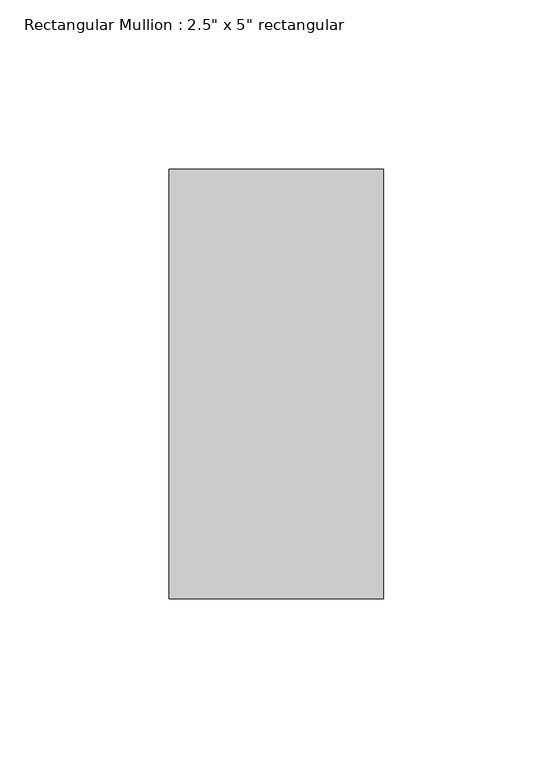
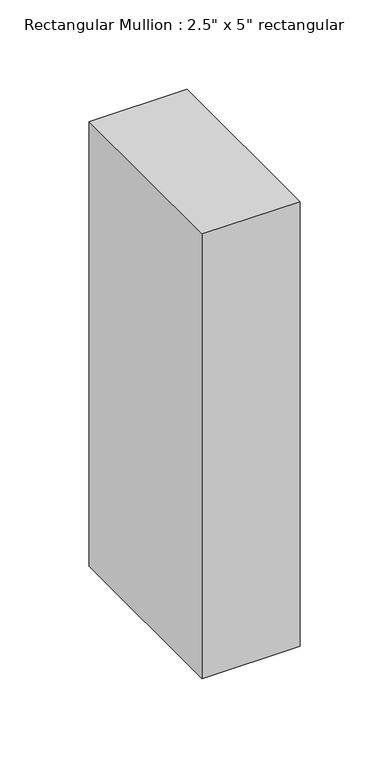
"""IFC4 building model written with IfcOpenShell, lengths in millimetres: member geometry."""

from ifc_helpers import new_model, si_unit, frame, origin, place, context, project, spatial, polyline, outline, extrude, source, transform, mapped, element, save


def member_3c3dc66a(model_context):
    return source(origin(), model_context, "Body", "SweptSolid", [
        extrude(outline(polyline([(0.0, 63.5), (0.0, -63.5), (-63.5, -63.5), (-63.5, 63.5), (0.0, 63.5)])), frame((0.0, 0.0, -304.8), z_axis=(0.0, 0.0, 1.0), x_axis=(1.0, 0.0, 0.0)), (0.0, 0.0, 1.0), 304.8),
    ])


if __name__ == "__main__":
    model = new_model("IFC4")
    model_context = context("Model", 3, world=origin())
    ifc_project = project(units=[si_unit("LENGTHUNIT", "METRE", prefix="MILLI")], contexts=[model_context])
    site = spatial("IfcSite", under=ifc_project)
    building = spatial("IfcBuilding", under=site)
    placement = place(None, origin())
    member_shape = member_3c3dc66a(model_context)
    element("IfcMember", 1, ObjectType="Rectangular Mullion : 2.5\" x 5\" rectangular", at=placement, inside=building, context=model_context, shape_type="MappedRepresentation", body=[
        mapped(member_shape, transform((0.0, 0.0, 0.0), x_axis=(1.0, 0.0, 0.0), y_axis=(0.0, 1.0, 0.0), z_axis=(0.0, 0.0, 1.0))),
    ])
    save(model, "model.ifc")

# Revit data of these elements
# Type "Rectangular Mullion : 2.5\" x 5\" rectangular"
#   built-in parameter 1007304 = 0.416667 (stored number, unit not read)
#   built-in parameter 1007301 = 0.104167 (stored number, unit not read)
#   built-in parameter 1007300 = 0.104167 (stored number, unit not read)
